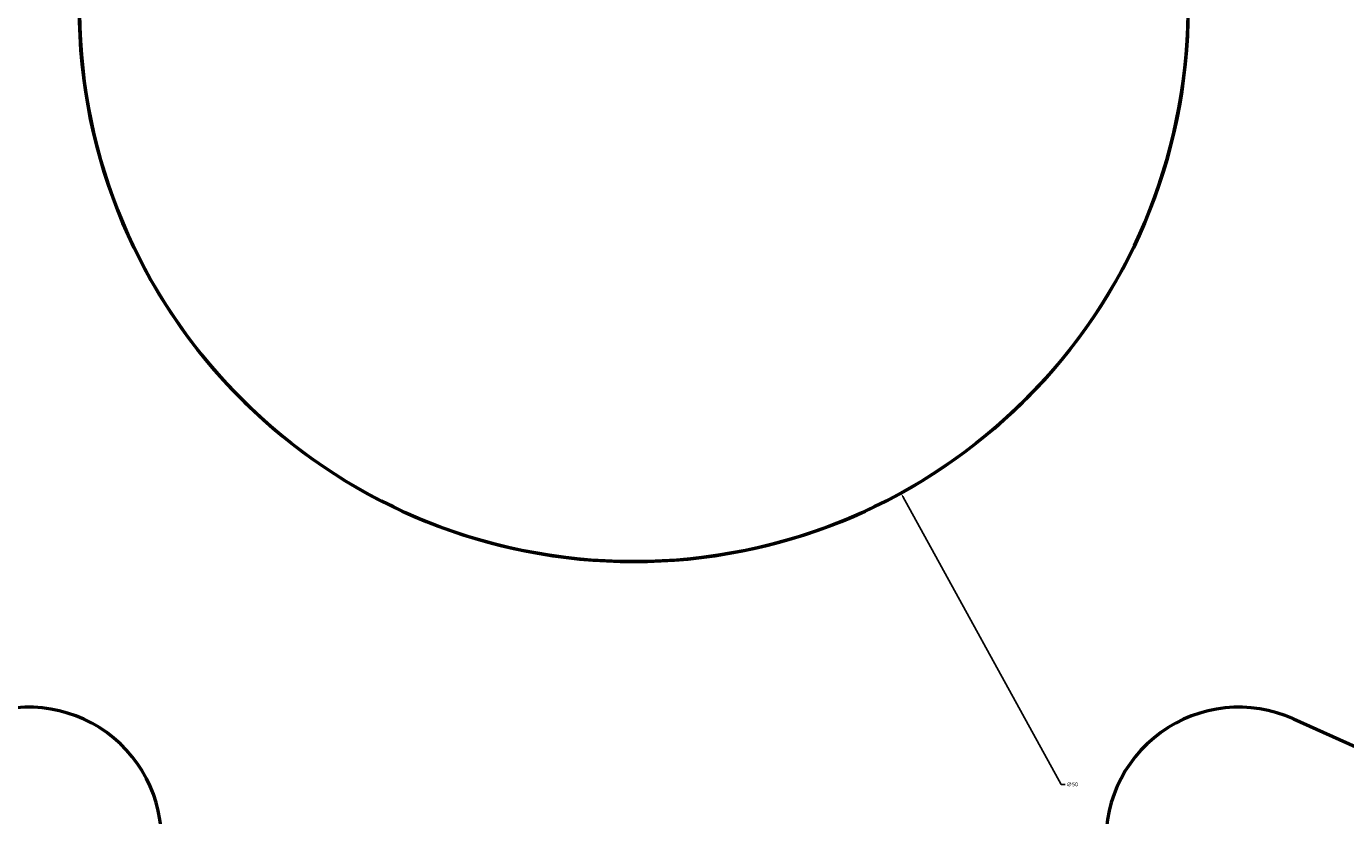
# Model space of a CAD drawing. Units: inches. Extents: x -99 to 284, y -92 to 134.
# Tile 3 of 16: x 5 to 64, y -22 to 14. Entities that reach past the tile are written whole.
import ezdxf

# ---------------------------------------------------------------- set-up
doc = ezdxf.new("R2010")
doc.units = ezdxf.units.IN
doc.header["$MEASUREMENT"] = 0
doc.layers.add('M-DIMS', color=2, linetype='Continuous', lineweight=18)
doc.layers.add('M-OUTL', color=7, linetype='Continuous', lineweight=50)
doc.styles.get("Standard").update_dxf_attribs({"font": 'arial.ttf'})
doc.dimstyles.get("Standard").update_dxf_attribs({"dimtxt": 0.18, "dimasz": 0.18, "dimexe": 0.18, "dimexo": 0.0625, "dimgap": 0.09, "dimtad": 0, "dimtih": 1, "dimtoh": 1, "dimdec": 4, "dimzin": 0, "dimdsep": 46, "dimtxsty": 'Standard', "dimcen": 0.09, "dimadec": 0, "dimazin": 0, "dimtfac": 1, "dimtdec": 4, "dimtofl": 0, "dimtmove": 0, "dimatfit": 3, "dimfxl": 1, "dimtolj": 1, "dimtzin": 0, "dimarcsym": 0})

# ---------------------------------------------------------------- blocks, each defined once
blk = doc.blocks.new('*U1')
for p, q in [((-5.205, -13.52), (-17.34, 7.646)), ((5.205, -13.52), (17.34, 7.646))]:
    blk.add_line(p, q)
for centre, start, end in [((-12.135, 10.63), 100.17697, 209.82635), ((12.135, 10.63), 330.17365, 79.82303), ((0, -10.536), 209.82635, 330.17365)]:
    blk.add_arc(centre, 6, start, end)
blk = doc.blocks.new('*U2')
at = {"layer": 'M-OUTL', "color": 0, "linetype": 'ByBlock', "lineweight": -2, "transparency": 16777216}
for p, rotation in [((-1.509, -31.235), 144), ((65.462, -31.235), 216)]:
    blk.add_blockref('*U1', p, dxfattribs=dict(at, rotation=rotation))
blk = doc.blocks.new('*D19')
at = {"layer": 'Defpoints', "color": 0, "transparency": 16777216}
for p in [(112.982, 51.721), (-49.029, -22.013)]:
    blk.add_point(p, dxfattribs=at)
at = {"layer": 'M-DIMS', "color": 0, "lineweight": -2, "transparency": 16777216}
for p, q in [((31.976, 14.764), (31.976, 14.944)), ((31.886, 14.854), (32.066, 14.854)), ((-97.632, -44.133), (-49.192, -22.088)), ((-97.812, -44.133), (-97.632, -44.133))]:
    blk.add_line(p, q, dxfattribs=at)
at = {"layer": 'M-DIMS', "color": 0, "transparency": 16777216}
blk.add_solid([(-49.205, -22.06), (-49.18, -22.115), (-49.029, -22.013)], dxfattribs=at)
at = {"layer": 'M-DIMS', "color": 0, "transparency": 16777216, "insert": (-98.199, -44.133), "char_height": 0.18, "attachment_point": 5}
blk.add_mtext('\\A1;∅178', dxfattribs=at)
blk = doc.blocks.new('*D20')
at = {"layer": 'Defpoints', "color": 0, "transparency": 16777216}
for p in [(-35.23, 65.245), (99.183, -35.537)]:
    blk.add_point(p, dxfattribs=at)
at = {"layer": 'M-DIMS', "color": 0, "lineweight": -2, "transparency": 16777216}
for p, q in [((31.976, 14.764), (31.976, 14.944)), ((31.886, 14.854), (32.066, 14.854)), ((139.507, -65.772), (99.327, -35.645)), ((139.687, -65.772), (139.507, -65.772))]:
    blk.add_line(p, q, dxfattribs=at)
at = {"layer": 'M-DIMS', "color": 0, "transparency": 16777216}
blk.add_solid([(99.345, -35.621), (99.309, -35.669), (99.183, -35.537)], dxfattribs=at)
at = {"layer": 'M-DIMS', "color": 0, "transparency": 16777216, "insert": (140.074, -65.772), "char_height": 0.18, "attachment_point": 5}
blk.add_mtext('\\A1;∅168', dxfattribs=at)
blk = doc.blocks.new('*D21')
at = {"layer": 'Defpoints', "color": 0, "transparency": 16777216}
for p in [(19.926, 36.758), (44.027, -7.05)]:
    blk.add_point(p, dxfattribs=at)
at = {"layer": 'M-DIMS', "color": 0, "lineweight": -2, "transparency": 16777216}
for p, q in [((31.976, 14.764), (31.976, 14.944)), ((31.886, 14.854), (32.066, 14.854)), ((51.258, -20.192), (44.114, -7.208)), ((51.438, -20.192), (51.258, -20.192))]:
    blk.add_line(p, q, dxfattribs=at)
at = {"layer": 'M-DIMS', "color": 0, "transparency": 16777216}
blk.add_solid([(44.14, -7.193), (44.088, -7.222), (44.027, -7.05)], dxfattribs=at)
at = {"layer": 'M-DIMS', "color": 0, "transparency": 16777216, "insert": (51.755, -20.192), "char_height": 0.18, "attachment_point": 5}
blk.add_mtext('\\A1;∅50', dxfattribs=at)

msp = doc.modelspace()

# ---------------------------------------------------------------- linework, layer by layer
at = {"layer": 'M-OUTL'}
for radius in [89, 84, 25]:
    msp.add_circle((31.9765, 14.8539), radius, dxfattribs=at)
msp.add_arc((31.9765, 14.8539), 25, 96.892103, 83.107897, dxfattribs=at)

# ---------------------------------------------------------------- block references
msp.add_blockref('*U2', (0, 0), dxfattribs=at)

# ---------------------------------------------------------------- dimensions: what is measured, and where the dimension line sits
at = {"layer": 'M-DIMS'}
for p1, p2, picture, middle in [((-35.2301, 65.2451), (99.1831, -35.5373), '*D20', (140.074, -65.772)), ((112.9816, 51.7208), (-49.0286, -22.013), '*D19', (-98.1987, -44.1332)), ((19.9255, 36.7577), (44.0274, -7.0499), '*D21', (51.7545, -20.1921))]:
    dim = msp.add_diameter_dim_2p(p1=p1, p2=p2, dimstyle='Standard', override={"dimdec": 0, "dimlfac": 1, "dimrnd": 0, "dimzin": 0, "dimdsep": 46, "dimlunit": 2}, dxfattribs=at)
    dim.commit()
    dim.dimension.update_dxf_attribs({"geometry": picture, "text_midpoint": middle, "dimtype": 163})

doc.saveas('drawing.dxf')
